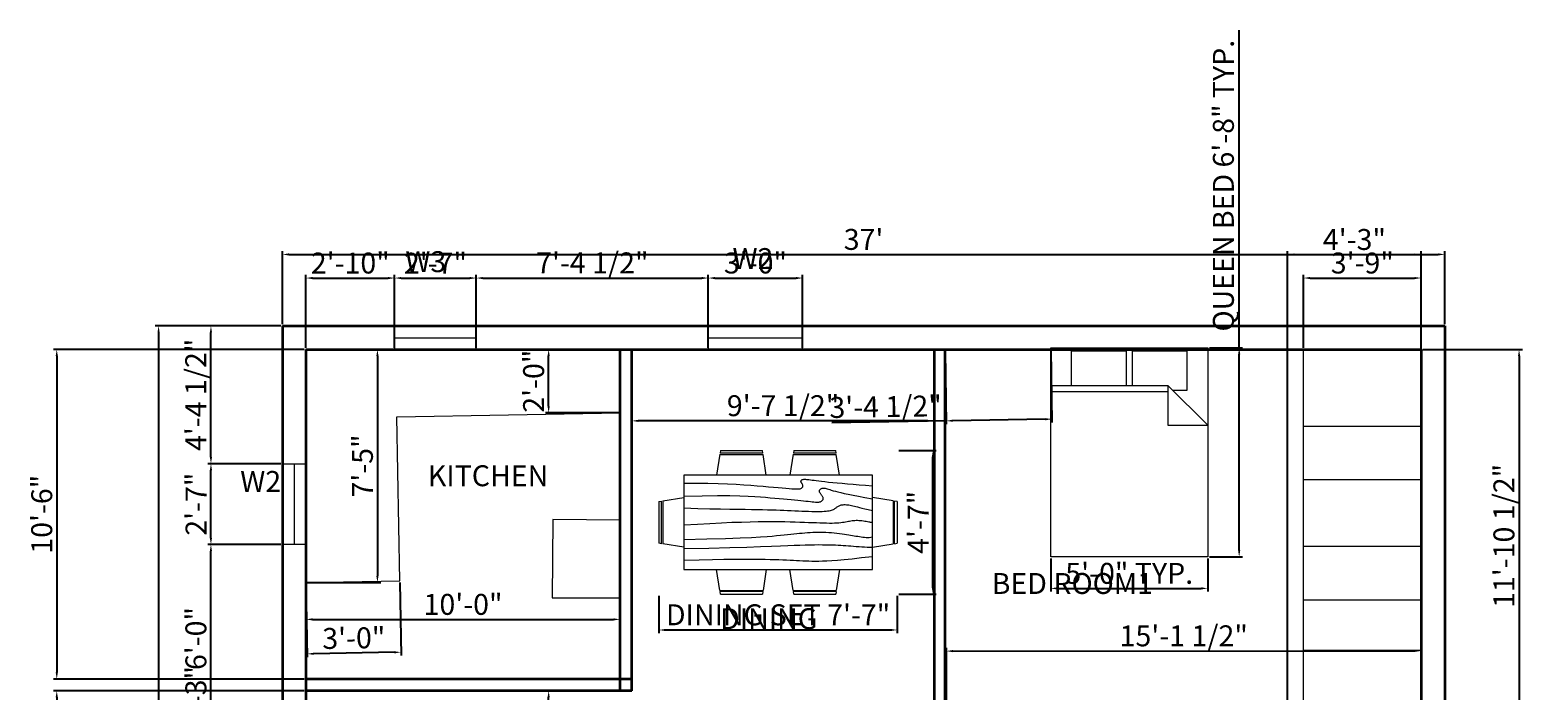
# Model space of a CAD drawing. Units: inches. Extents: x 56 to 631, y 587 to 1198.
# Tile 3 of 3: x 56 to 631, y 946 to 1198. Entities that reach past the tile are written whole.
import ezdxf

# ---------------------------------------------------------------- set-up
doc = ezdxf.new("R2010")
doc.units = ezdxf.units.IN
for name, color, linetype, lineweight in [('A-ANNO-DIMS', 2, 'Continuous', 18), ('A-ANNO-TEXT', 7, 'Continuous', 18), ('A-AREA-IDEN', 7, 'Continuous', 25), ('A-FLOR-CASE', 9, 'Continuous', 18), ('A-FURN', 8, 'Continuous', 18), ('A-GLAZ', 4, 'Continuous', 18), ('WALL', 7, 'Continuous', 35)]:
    doc.layers.add(name, color=color, linetype=linetype, lineweight=lineweight)
doc.styles.get("Standard").update_dxf_attribs({"font": 'arial.ttf', "height": 8})
doc.dimstyles.new('ISO-25', dxfattribs={"dimtxt": 2.5, "dimasz": 2.5, "dimexe": 1.25, "dimexo": 0.625, "dimtad": 1, "dimdec": 1, "dimlunit": 3, "dimtxsty": 'Standard', "dimcen": 2.5, "dimadec": 0, "dimazin": 0, "dimtfac": 1, "dimtdec": 1, "dimtmove": 0, "dimatfit": 3, "dimfxl": 1, "dimarcsym": 0})

# ---------------------------------------------------------------- blocks, each defined once
blk = doc.blocks.new('Dining Set - 36 x 72 in.')
for p, q in [((-22.2343, 26.00059), (-23.4847, 17.99762)), ((-22.2304, 26), (-5.7608, 26)), ((-22, 27.5), (-22.1562, 26.50042)), ((-5.8416, 26.5), (-22.1534, 26.5)), ((-22, 27.5), (-6, 27.5)), ((-5.8437, 26.49966), (-6, 27.5)), ((-4.5152, 17.99762), (-5.7655, 25.99926)), ((5.7657, 26.00059), (4.5153, 17.99762)), ((5.7696, 26), (22.2392, 26)), ((6, 27.5), (5.8438, 26.50042)), ((22.1584, 26.5), (5.8466, 26.5)), ((6, 27.5), (22, 27.5)), ((22.1563, 26.49966), (22, 27.5)), ((23.4848, 17.99762), (22.2345, 25.99926)), ((36, 18), (-36, 18)), ((-36, 18), (-36, -18)), ((36, -18), (36, 18)), ((-45.5, 8), (-44.5004, 8.15617)), ((-45.5, 8), (-45.5, -8)), ((-44.5, -8.15843), (-44.5, 8.15338)), ((-44.0006, 8.23428), (-35.9976, 9.48474)), ((-44, 8.23041), (-44, -8.23915)), ((44.0006, 8.23428), (35.9976, 9.48474)), ((44, 8.23041), (44, -8.23915)), ((44.5, -8.15843), (44.5, 8.15338)), ((45.5, 8), (44.5005, 8.15617)), ((45.5, 8), (45.5, -8)), ((-44.4997, -8.15631), (-45.5, -8)), ((-35.9976, -9.48476), (-43.9993, -8.2345)), ((35.9976, -9.48476), (43.9993, -8.2345)), ((44.4997, -8.15631), (45.5, -8)), ((-36, -18), (36, -18)), ((-22.2343, -26.0006), (-23.4847, -17.99762)), ((-4.5152, -17.99762), (-5.7655, -25.99928)), ((5.7657, -26.0006), (4.5153, -17.99762)), ((23.4848, -17.99762), (22.2345, -25.99928)), ((-22.2304, -26), (-5.7608, -26)), ((-22, -27.5), (-22.1562, -26.50044)), ((-5.8416, -26.5), (-22.1534, -26.5)), ((-22, -27.5), (-6, -27.5)), ((-5.8437, -26.49967), (-6, -27.5)), ((5.7696, -26), (22.2392, -26)), ((6, -27.5), (5.8438, -26.50044)), ((22.1584, -26.5), (5.8466, -26.5)), ((6, -27.5), (22, -27.5)), ((22.1563, -26.49967), (22, -27.5))]:
    blk.add_line(p, q)
for points in [[(-36, 15), (-31.1772, 14.97754), (-26.8079, 14.91406), (-22.8538, 14.81543), (-19.276, 14.6875), (-16.0362, 14.53613), (-13.0957, 14.36718), (-10.4159, 14.18652), (-7.9583, 14), (-5.6904, 13.81315), (-3.6035, 13.63021), (-1.6954, 13.45508), (0.0365, 13.29166), (1.5945, 13.14388), (2.9811, 13.01562), (4.1988, 12.9108), (5.25, 12.83333), (6.1393, 12.78613), (6.8802, 12.76823), (7.4883, 12.77767), (7.9792, 12.8125), (8.3685, 12.87077), (8.6719, 12.95052), (8.9049, 13.0498), (9.0833, 13.16666), (9.2205, 13.29899), (9.3216, 13.44401), (9.3895, 13.59879), (9.4271, 13.76041), (9.4373, 13.92594), (9.4232, 14.09245), (9.3875, 14.257), (9.3333, 14.41666), (9.2638, 14.56917), (9.1836, 14.71484), (9.0975, 14.85465), (9.0104, 14.98958), (8.9272, 15.1206), (8.8529, 15.2487), (8.7922, 15.37483), (8.75, 15.5), (8.7305, 15.62467), (8.7344, 15.74739), (8.7617, 15.86621), (8.8125, 15.97916), (8.8867, 16.08431), (8.9844, 16.17968), (9.1055, 16.26334), (9.25, 16.33333), (9.4189, 16.38802), (9.6172, 16.42708), (9.8506, 16.45052), (10.125, 16.45833), (10.4463, 16.45052), (10.8203, 16.42708), (11.2529, 16.38802), (11.75, 16.33333), (12.3184, 16.26318), (12.9694, 16.17838), (13.7151, 16.07991), (14.5677, 15.96875), (15.5395, 15.84586), (16.6426, 15.71224), (17.8893, 15.56884), (19.2917, 15.41666), (20.859, 15.25667), (22.5879, 15.08984), (24.4721, 14.91715), (26.5052, 14.73958), (28.6809, 14.5581), (30.9929, 14.3737), (33.4347, 14.18733), (36, 14)], [(-36, 10), (-28.9766, 10.14274), (-23.1725, 10.20442), (-18.4241, 10.19775), (-14.5677, 10.13541), (-11.4399, 10.03011), (-8.877, 9.89453), (-6.7154, 9.74137), (-4.7917, 9.58333), (-2.9698, 9.43082), (-1.2246, 9.28515), (0.4415, 9.14534), (2.026, 9.01041), (3.5266, 8.87939), (4.9408, 8.7513), (6.266, 8.62516), (7.5, 8.5), (8.6411, 8.37549), (9.6914, 8.2539), (10.6538, 8.13818), (11.5312, 8.03125), (12.3267, 7.93603), (13.043, 7.85547), (13.6831, 7.79248), (14.25, 7.75), (14.7471, 7.7303), (15.1797, 7.73307), (15.5537, 7.75732), (15.875, 7.80208), (16.1494, 7.86637), (16.3828, 7.94922), (16.5811, 8.04964), (16.75, 8.16666), (16.8944, 8.29915), (17.0143, 8.44531), (17.1089, 8.60319), (17.1771, 8.77083), (17.218, 8.94629), (17.2305, 9.1276), (17.2137, 9.31282), (17.1667, 9.5), (17.0895, 9.6875), (16.987, 9.875), (16.8649, 10.0625), (16.7292, 10.25), (16.5856, 10.4375), (16.4401, 10.625), (16.2985, 10.8125), (16.1667, 11), (16.05, 11.18733), (15.9518, 11.3737), (15.8752, 11.5581), (15.8229, 11.73958), (15.798, 11.91715), (15.8034, 12.08984), (15.842, 12.25667), (15.9167, 12.41666), (16.0295, 12.56836), (16.1784, 12.70833), (16.3605, 12.83268), (16.5729, 12.9375), (16.8127, 13.01888), (17.0768, 13.07291), (17.3625, 13.0957), (17.6667, 13.08333), (17.9894, 13.03312), (18.3418, 12.94726), (18.7382, 12.82918), (19.1927, 12.68229), (19.7195, 12.51001), (20.3327, 12.31575), (21.0465, 12.10294), (21.875, 11.875), (22.8357, 11.63354), (23.959, 11.37304), (25.2786, 11.08618), (26.8282, 10.76562), (28.6414, 10.40405), (30.752, 9.99414), (33.1936, 9.52856), (36, 9)], [(-36, 5.5), (-30.7157, 5.3348), (-26.069, 5.20963), (-21.9946, 5.11767), (-18.4271, 5.05208), (-15.3009, 5.00602), (-12.5508, 4.97265), (-10.1112, 4.94515), (-7.9167, 4.91666), (-5.909, 4.88167), (-4.0586, 4.83984), (-2.3429, 4.79215), (-0.7396, 4.73958), (0.7739, 4.6831), (2.22, 4.6237), (3.6213, 4.56233), (5, 4.5), (6.373, 4.43782), (7.7344, 4.3776), (9.0723, 4.32129), (10.375, 4.27083), (11.6309, 4.22819), (12.8281, 4.19531), (13.9551, 4.17415), (15, 4.16666), (15.954, 4.17448), (16.819, 4.19791), (17.6001, 4.23698), (18.3021, 4.29166), (18.9299, 4.36198), (19.4883, 4.44791), (19.9823, 4.54948), (20.4167, 4.66666), (20.7969, 4.79899), (21.1302, 4.94401), (21.4245, 5.09879), (21.6875, 5.26041), (21.9271, 5.42594), (22.1511, 5.59245), (22.3672, 5.757), (22.5834, 5.91666), (22.8065, 6.06868), (23.0404, 6.21093), (23.2879, 6.34147), (23.5521, 6.45833), (23.8358, 6.55957), (24.142, 6.64323), (24.4735, 6.70735), (24.8334, 6.75), (25.2235, 6.76969), (25.642, 6.76692), (26.0858, 6.74267), (26.5521, 6.69791), (27.0379, 6.63362), (27.5404, 6.55078), (28.0565, 6.45036), (28.5834, 6.33333), (29.1242, 6.19987), (29.7071, 6.04687), (30.3661, 5.87044), (31.1354, 5.66666), (32.0493, 5.43164), (33.142, 5.16146), (34.4475, 4.85221), (36, 4.5)], [(-36, -1), (-30.7915, -0.6591), (-26.0195, -0.38216), (-21.6519, -0.16284), (-17.6563, 0.00521), (-14.0005, 0.12833), (-10.6523, 0.21289), (-7.5796, 0.26522), (-4.75, 0.29166), (-2.134, 0.29793), (0.2878, 0.28711), (2.5317, 0.26163), (4.6146, 0.22396), (6.5529, 0.17651), (8.3633, 0.12174), (10.0623, 0.06209), (11.6667, 0), (13.1899, -0.06201), (14.6341, -0.1211), (15.9982, -0.17432), (17.2813, -0.21875), (18.4823, -0.25147), (19.6003, -0.26953), (20.6343, -0.27002), (21.5834, -0.25), (22.4481, -0.20768), (23.2357, -0.14584), (23.9549, -0.06836), (24.6146, 0.02083), (25.2235, 0.11784), (25.7904, 0.21875), (26.3241, 0.31966), (26.8334, 0.41666), (27.3265, 0.50618), (27.8099, 0.58593), (28.2894, 0.65397), (28.7709, 0.70833), (29.2601, 0.74707), (29.763, 0.76823), (30.2855, 0.76985), (30.8334, 0.75), (31.4088, 0.70784), (31.9994, 0.64713), (32.589, 0.57275), (33.1615, 0.48958), (33.7008, 0.4025), (34.1908, 0.3164), (34.6153, 0.23616), (34.9584, 0.16666), (35.2099, 0.11165), (35.3848, 0.07031), (35.504, 0.04069), (35.5886, 0.02083), (35.6594, 0.00879), (35.7377, 0.0026), (35.8442, 0.00032), (36, 0)], [(-36, -6.5), (-27.1843, -6.31267), (-20.084, -6.1263), (-14.469, -5.9419), (-10.1094, -5.76042), (-6.7752, -5.58285), (-4.2363, -5.41016), (-2.2629, -5.24333), (-0.625, -5.08334), (0.8708, -4.93099), (2.2715, -4.78646), (3.5872, -4.64974), (4.8281, -4.52084), (6.0046, -4.39974), (7.127, -4.28646), (8.2053, -4.18099), (9.25, -4.08334), (10.2705, -3.99382), (11.2734, -3.91407), (12.2647, -3.84603), (13.25, -3.79167), (14.2354, -3.75293), (15.2266, -3.73177), (16.2295, -3.73015), (17.25, -3.75), (18.2912, -3.79248), (19.3451, -3.85547), (20.4009, -3.93604), (21.4479, -4.03125), (22.4754, -4.13819), (23.4727, -4.25391), (24.4289, -4.37549), (25.3334, -4.5), (26.1785, -4.62492), (26.9694, -4.74935), (27.7145, -4.87281), (28.4219, -4.99479), (29.1, -5.11483), (29.7572, -5.23242), (30.4016, -5.34709), (31.0417, -5.45834), (31.6837, -5.56437), (32.3262, -5.65821), (32.9658, -5.73153), (33.599, -5.77604), (34.2224, -5.78345), (34.8327, -5.74545), (35.4264, -5.65373), (36, -5.5)], [(-36, -10), (-26.4022, -9.81299), (-18.4675, -9.62891), (-11.9839, -9.45069), (-6.7396, -9.28125), (-2.5226, -9.12354), (0.8789, -8.98047), (3.6769, -8.85498), (6.0833, -8.75), (8.2767, -8.66765), (10.3021, -8.60677), (12.1712, -8.56543), (13.8958, -8.54167), (15.4876, -8.53353), (16.9583, -8.53907), (18.3197, -8.55632), (19.5834, -8.58334), (20.7616, -8.61841), (21.8685, -8.66081), (22.9188, -8.71004), (23.9271, -8.76563), (24.9081, -8.82707), (25.8763, -8.89388), (26.8465, -8.96558), (27.8334, -9.04167), (28.8474, -9.12118), (29.8828, -9.20117), (30.93, -9.27824), (31.9792, -9.34896), (33.0205, -9.40991), (34.0443, -9.45768), (35.0407, -9.48885), (36, -9.5)], [(-36, -14.5), (-30.0881, -14.33513), (-25.0332, -14.21224), (-20.7312, -14.12647), (-17.0781, -14.07292), (-13.97, -14.04671), (-11.3027, -14.04297), (-8.9724, -14.05681), (-6.875, -14.08334), (-4.9224, -14.11833), (-3.0905, -14.16016), (-1.3709, -14.20785), (0.2448, -14.26042), (1.7647, -14.3169), (3.1973, -14.3763), (4.5507, -14.43767), (5.8333, -14.5), (7.0554, -14.5621), (8.235, -14.62175), (9.3922, -14.67652), (10.5469, -14.72396), (11.7192, -14.76164), (12.929, -14.78711), (14.1965, -14.79794), (15.5417, -14.79167), (16.9933, -14.76424), (18.6152, -14.70508), (20.4804, -14.60197), (22.6615, -14.44271), (25.2312, -14.21509), (28.2624, -13.9069), (31.8277, -13.50594), (36, -13)]]:
    blk.add_lwpolyline(points)
blk = doc.blocks.new('Bed - Queen')
for p, q in [((0, -80.00003), (0, 0)), ((0, 0), (59.99999, 0)), ((59.99999, 0), (59.99999, -80.00003)), ((7.99999, -1.2), (28.79998, -1.2)), ((7.99999, -14.4), (7.99999, -1.2)), ((28.79998, -1.2), (28.79998, -14.4)), ((31.19999, -1.2), (51.99999, -1.2)), ((31.19999, -14.4), (31.19999, -1.2)), ((51.99999, -1.2), (51.99999, -16.4)), ((0, -14.4), (44.8, -14.4)), ((44.8, -16.8), (0, -16.8)), ((59.99999, -29.6), (44.8, -14.4)), ((44.8, -14.4), (44.8, -29.6)), ((51.99999, -16.4), (46.79936, -16.4)), ((44.8, -29.6), (59.99999, -29.6)), ((59.99999, -80.00003), (0, -80.00003))]:
    blk.add_line(p, q)
blk = doc.blocks.new('*D11')
at = {"layer": 'A-ANNO-DIMS', "color": 0, "lineweight": -2, "transparency": 16777216}
for p, q in [((151.92, 1085.91), (151.92, 1113.87)), ((154.42, 1112.62), (593.42, 1112.62)), ((595.92, 1085.91), (595.92, 1113.87))]:
    blk.add_line(p, q, dxfattribs=at)
at = {"layer": 'A-ANNO-DIMS', "color": 0, "transparency": 16777216}
for points in [[(154.42, 1113.04), (154.42, 1112.2), (151.92, 1112.62)], [(593.42, 1113.04), (593.42, 1112.2), (595.92, 1112.62)]]:
    blk.add_solid(points, dxfattribs=at)
at = {"layer": 'Defpoints', "color": 0, "transparency": 16777216}
for p in [(595.92, 1112.62), (151.92, 1085.29), (595.92, 1085.29)]:
    blk.add_point(p, dxfattribs=at)
at = {"layer": 'A-ANNO-DIMS', "color": 0, "transparency": 16777216, "insert": (373.92, 1117.33), "char_height": 8, "attachment_point": 5}
blk.add_mtext("37'", dxfattribs=at)
blk = doc.blocks.new('*D12')
at = {"layer": 'A-ANNO-DIMS', "color": 0, "lineweight": -2, "transparency": 16777216}
for p, q in [((151.29, 1085.29), (103.37, 1085.29)), ((104.62, 1082.79), (104.62, 624.29)), ((151.29, 621.79), (103.37, 621.79))]:
    blk.add_line(p, q, dxfattribs=at)
at = {"layer": 'A-ANNO-DIMS', "color": 0, "transparency": 16777216}
for points in [[(104.2, 1082.79), (105.03, 1082.79), (104.62, 1085.29)], [(104.2, 624.29), (105.03, 624.29), (104.62, 621.79)]]:
    blk.add_solid(points, dxfattribs=at)
at = {"layer": 'Defpoints', "color": 0, "transparency": 16777216}
for p in [(151.92, 1085.29), (104.62, 621.79), (151.92, 621.79)]:
    blk.add_point(p, dxfattribs=at)
at = {"layer": 'A-ANNO-DIMS', "color": 0, "transparency": 16777216, "insert": (99.9, 853.54), "char_height": 8, "attachment_point": 5, "rotation": 90}
blk.add_mtext('38\'-7.5"', dxfattribs=at)
blk = doc.blocks.new('*D13')
at = {"layer": 'A-ANNO-DIMS', "color": 0, "lineweight": -2, "transparency": 16777216}
for p, q in [((517.4, 1076.94), (517.4, 1198.37)), ((506.03, 1076.94), (518.65, 1076.94)), ((517.4, 999.44), (517.4, 1074.44)), ((506.03, 996.94), (518.65, 996.94))]:
    blk.add_line(p, q, dxfattribs=at)
at = {"layer": 'A-ANNO-DIMS', "color": 0, "transparency": 16777216}
for points in [[(516.99, 1074.44), (517.82, 1074.44), (517.4, 1076.94)], [(516.99, 999.44), (517.82, 999.44), (517.4, 996.94)]]:
    blk.add_solid(points, dxfattribs=at)
at = {"layer": 'Defpoints', "color": 0, "transparency": 16777216}
for p in [(505.4, 1076.94), (517.4, 1076.94), (505.4, 996.94)]:
    blk.add_point(p, dxfattribs=at)
at = {"layer": 'A-ANNO-DIMS', "color": 0, "transparency": 16777216, "insert": (512.4, 1138.91), "char_height": 8, "attachment_point": 5, "rotation": 90}
blk.add_mtext('QUEEN BED 6\'-8" TYP.', dxfattribs=at)
blk = doc.blocks.new('*D14')
at = {"layer": 'A-ANNO-DIMS', "color": 0, "lineweight": -2, "transparency": 16777216}
for p, q in [((445.4, 996.32), (445.4, 983.69)), ((505.4, 996.32), (505.4, 983.69)), ((447.9, 984.94), (502.9, 984.94))]:
    blk.add_line(p, q, dxfattribs=at)
at = {"layer": 'A-ANNO-DIMS', "color": 0, "transparency": 16777216}
for points in [[(447.9, 985.36), (447.9, 984.53), (445.4, 984.94)], [(502.9, 985.36), (502.9, 984.53), (505.4, 984.94)]]:
    blk.add_solid(points, dxfattribs=at)
at = {"layer": 'Defpoints', "color": 0, "transparency": 16777216}
for p in [(445.4, 996.94), (505.4, 996.94), (505.4, 984.94)]:
    blk.add_point(p, dxfattribs=at)
at = {"layer": 'A-ANNO-DIMS', "color": 0, "transparency": 16777216, "insert": (475.4, 989.65), "char_height": 8, "attachment_point": 5}
blk.add_mtext('5\'-0" TYP.', dxfattribs=at)
blk = doc.blocks.new('*D15')
at = {"layer": 'A-ANNO-DIMS', "color": 0, "lineweight": -2, "transparency": 16777216}
for p, q in [((295.77, 982.06), (295.77, 967.79)), ((386.77, 982.06), (386.77, 967.79)), ((298.27, 969.04), (384.27, 969.04))]:
    blk.add_line(p, q, dxfattribs=at)
at = {"layer": 'A-ANNO-DIMS', "color": 0, "transparency": 16777216}
for points in [[(298.27, 969.45), (298.27, 968.62), (295.77, 969.04)], [(384.27, 969.45), (384.27, 968.62), (386.77, 969.04)]]:
    blk.add_solid(points, dxfattribs=at)
at = {"layer": 'Defpoints', "color": 0, "transparency": 16777216}
for p in [(295.77, 982.69), (386.77, 982.69), (386.77, 969.04)]:
    blk.add_point(p, dxfattribs=at)
at = {"layer": 'A-ANNO-DIMS', "color": 0, "transparency": 16777216, "insert": (341.27, 973.8), "char_height": 8, "attachment_point": 5}
blk.add_mtext('DINING SET 7\'-7"', dxfattribs=at)
blk = doc.blocks.new('*D16')
at = {"layer": 'A-ANNO-DIMS', "color": 0, "lineweight": -2, "transparency": 16777216}
for p, q in [((387.39, 1037.69), (401.67, 1037.69)), ((400.42, 985.19), (400.42, 1035.19)), ((387.39, 982.69), (401.67, 982.69))]:
    blk.add_line(p, q, dxfattribs=at)
at = {"layer": 'A-ANNO-DIMS', "color": 0, "transparency": 16777216}
for points in [[(400, 1035.19), (400.84, 1035.19), (400.42, 1037.69)], [(400, 985.19), (400.84, 985.19), (400.42, 982.69)]]:
    blk.add_solid(points, dxfattribs=at)
at = {"layer": 'Defpoints', "color": 0, "transparency": 16777216}
for p in [(386.77, 1037.69), (400.42, 1037.69), (386.77, 982.69)]:
    blk.add_point(p, dxfattribs=at)
at = {"layer": 'A-ANNO-DIMS', "color": 0, "transparency": 16777216, "insert": (395.79, 1010.19), "char_height": 8, "attachment_point": 5, "rotation": 90}
blk.add_mtext('4\'-7"', dxfattribs=at)
blk = doc.blocks.new('*D22')
at = {"layer": 'A-ANNO-DIMS', "color": 0, "lineweight": -2, "transparency": 16777216}
for p, q in [((160.92, 946.41), (160.92, 974.34)), ((280.92, 946.41), (280.92, 974.34)), ((163.42, 973.09), (278.42, 973.09))]:
    blk.add_line(p, q, dxfattribs=at)
at = {"layer": 'A-ANNO-DIMS', "color": 0, "transparency": 16777216}
for points in [[(163.42, 973.5), (163.42, 972.67), (160.92, 973.09)], [(278.42, 973.5), (278.42, 972.67), (280.92, 973.09)]]:
    blk.add_solid(points, dxfattribs=at)
at = {"layer": 'Defpoints', "color": 0, "transparency": 16777216}
for p in [(280.92, 973.09), (160.92, 945.79), (280.92, 945.79)]:
    blk.add_point(p, dxfattribs=at)
at = {"layer": 'A-ANNO-DIMS', "color": 0, "transparency": 16777216, "insert": (220.92, 977.79), "char_height": 8, "attachment_point": 5}
blk.add_mtext('10\'-0"', dxfattribs=at)
blk = doc.blocks.new('*D23')
at = {"layer": 'A-ANNO-DIMS', "color": 0, "lineweight": -2, "transparency": 16777216}
for p, q in [((285.42, 1075.66), (285.42, 1047.74)), ((400.92, 1075.66), (400.92, 1047.74)), ((398.42, 1048.99), (287.92, 1048.99))]:
    blk.add_line(p, q, dxfattribs=at)
at = {"layer": 'A-ANNO-DIMS', "color": 0, "transparency": 16777216}
for points in [[(287.92, 1049.4), (287.92, 1048.57), (285.42, 1048.99)], [(398.42, 1049.4), (398.42, 1048.57), (400.92, 1048.99)]]:
    blk.add_solid(points, dxfattribs=at)
at = {"layer": 'Defpoints', "color": 0, "transparency": 16777216}
for p in [(285.42, 1076.29), (400.92, 1076.29), (285.42, 1048.99)]:
    blk.add_point(p, dxfattribs=at)
at = {"layer": 'A-ANNO-DIMS', "color": 0, "transparency": 16777216, "insert": (343.17, 1053.75), "char_height": 8, "attachment_point": 5}
blk.add_mtext('9\'-7 1/2"', dxfattribs=at)
blk = doc.blocks.new('*D24')
at = {"layer": 'A-ANNO-DIMS', "color": 0, "lineweight": -2, "transparency": 16777216}
for p, q in [((405.55, 934.28), (405.54, 962.2)), ((586.91, 934.37), (586.9, 962.3)), ((408.04, 960.95), (584.4, 961.04))]:
    blk.add_line(p, q, dxfattribs=at)
at = {"layer": 'A-ANNO-DIMS', "color": 0, "transparency": 16777216}
for points in [[(408.04, 961.37), (408.04, 960.54), (405.54, 960.95)], [(584.4, 961.46), (584.4, 960.63), (586.9, 961.05)]]:
    blk.add_solid(points, dxfattribs=at)
at = {"layer": 'Defpoints', "color": 0, "transparency": 16777216}
for p in [(586.9, 961.05), (405.55, 933.65), (586.92, 933.75)]:
    blk.add_point(p, dxfattribs=at)
at = {"layer": 'A-ANNO-DIMS', "color": 0, "transparency": 16777216, "insert": (496.22, 965.76), "char_height": 8, "attachment_point": 5, "rotation": 0.02972}
blk.add_mtext('15\'-1 1/2"', dxfattribs=at)
blk = doc.blocks.new('*D26')
at = {"layer": 'A-ANNO-DIMS', "color": 0, "lineweight": -2, "transparency": 16777216}
for p, q in [((535.92, 796.41), (535.92, 1113.84)), ((538.42, 1112.59), (584.42, 1112.59)), ((586.92, 796.41), (586.92, 1113.84))]:
    blk.add_line(p, q, dxfattribs=at)
at = {"layer": 'A-ANNO-DIMS', "color": 0, "transparency": 16777216}
for points in [[(538.42, 1113), (538.42, 1112.17), (535.92, 1112.59)], [(584.42, 1113), (584.42, 1112.17), (586.92, 1112.59)]]:
    blk.add_solid(points, dxfattribs=at)
at = {"layer": 'Defpoints', "color": 0, "transparency": 16777216}
for p in [(586.92, 1112.59), (535.92, 795.79), (586.92, 795.79)]:
    blk.add_point(p, dxfattribs=at)
at = {"layer": 'A-ANNO-DIMS', "color": 0, "transparency": 16777216, "insert": (561.42, 1117.3), "char_height": 8, "attachment_point": 5}
blk.add_mtext('4\'-3"', dxfattribs=at)
blk = doc.blocks.new('*D27')
at = {"layer": 'A-ANNO-DIMS', "color": 0, "lineweight": -2, "transparency": 16777216}
for p, q in [((160.29, 1076.29), (64.47, 1076.29)), ((65.72, 1073.79), (65.72, 952.79)), ((160.29, 950.29), (64.47, 950.29))]:
    blk.add_line(p, q, dxfattribs=at)
at = {"layer": 'A-ANNO-DIMS', "color": 0, "transparency": 16777216}
for points in [[(65.31, 1073.79), (66.14, 1073.79), (65.72, 1076.29)], [(65.31, 952.79), (66.14, 952.79), (65.72, 950.29)]]:
    blk.add_solid(points, dxfattribs=at)
at = {"layer": 'Defpoints', "color": 0, "transparency": 16777216}
for p in [(160.92, 1076.29), (65.72, 950.29), (160.92, 950.29)]:
    blk.add_point(p, dxfattribs=at)
at = {"layer": 'A-ANNO-DIMS', "color": 0, "transparency": 16777216, "insert": (61.01, 1013.29), "char_height": 8, "attachment_point": 5, "rotation": 90}
blk.add_mtext('10\'-6"', dxfattribs=at)
blk = doc.blocks.new('*D28')
at = {"layer": 'A-ANNO-DIMS', "color": 0, "lineweight": -2, "transparency": 16777216}
for p, q in [((160.29, 945.79), (64.47, 945.79)), ((65.72, 943.29), (65.72, 900.29)), ((160.29, 897.79), (64.47, 897.79))]:
    blk.add_line(p, q, dxfattribs=at)
at = {"layer": 'A-ANNO-DIMS', "color": 0, "transparency": 16777216}
for points in [[(65.31, 943.29), (66.14, 943.29), (65.72, 945.79)], [(65.31, 900.29), (66.14, 900.29), (65.72, 897.79)]]:
    blk.add_solid(points, dxfattribs=at)
at = {"layer": 'Defpoints', "color": 0, "transparency": 16777216}
for p in [(160.92, 945.79), (65.72, 897.79), (160.92, 897.79)]:
    blk.add_point(p, dxfattribs=at)
at = {"layer": 'A-ANNO-DIMS', "color": 0, "transparency": 16777216, "insert": (61.01, 921.79), "char_height": 8, "attachment_point": 5, "rotation": 90}
blk.add_mtext('4\'-0"', dxfattribs=at)
blk = doc.blocks.new('*D30')
at = {"layer": 'A-ANNO-DIMS', "color": 0, "lineweight": -2, "transparency": 16777216}
for p, q in [((587.54, 1076.29), (625.57, 1076.29)), ((624.32, 1073.79), (624.32, 936.25)), ((587.54, 933.75), (625.57, 933.75))]:
    blk.add_line(p, q, dxfattribs=at)
at = {"layer": 'A-ANNO-DIMS', "color": 0, "transparency": 16777216}
for points in [[(623.9, 1073.79), (624.74, 1073.79), (624.32, 1076.29)], [(623.9, 936.25), (624.74, 936.25), (624.32, 933.75)]]:
    blk.add_solid(points, dxfattribs=at)
at = {"layer": 'Defpoints', "color": 0, "transparency": 16777216}
for p in [(586.92, 1076.29), (586.92, 933.75), (624.32, 933.75)]:
    blk.add_point(p, dxfattribs=at)
at = {"layer": 'A-ANNO-DIMS', "color": 0, "transparency": 16777216, "insert": (619.56, 1005.02), "char_height": 8, "attachment_point": 5, "rotation": 90}
blk.add_mtext('11\'-10 1/2"', dxfattribs=at)
blk = doc.blocks.new('*D33')
at = {"layer": 'A-ANNO-DIMS', "color": 0, "lineweight": -2, "transparency": 16777216}
for p, q in [((160.92, 1076.91), (160.92, 1104.84)), ((163.42, 1103.59), (192.28, 1103.59)), ((194.78, 1076.91), (194.78, 1104.84))]:
    blk.add_line(p, q, dxfattribs=at)
at = {"layer": 'A-ANNO-DIMS', "color": 0, "transparency": 16777216}
for points in [[(163.42, 1104), (163.42, 1103.17), (160.92, 1103.59)], [(192.28, 1104), (192.28, 1103.17), (194.78, 1103.59)]]:
    blk.add_solid(points, dxfattribs=at)
at = {"layer": 'Defpoints', "color": 0, "transparency": 16777216}
for p in [(194.78, 1103.59), (160.92, 1076.29), (194.78, 1076.29)]:
    blk.add_point(p, dxfattribs=at)
at = {"layer": 'A-ANNO-DIMS', "color": 0, "transparency": 16777216, "insert": (177.85, 1108.29), "char_height": 8, "attachment_point": 5}
blk.add_mtext('2\'-10"', dxfattribs=at)
blk = doc.blocks.new('*D34')
at = {"layer": 'A-ANNO-DIMS', "color": 0, "lineweight": -2, "transparency": 16777216}
for p, q in [((194.78, 1076.91), (194.78, 1104.84)), ((197.28, 1103.59), (223.48, 1103.59)), ((225.98, 1076.91), (225.98, 1104.84))]:
    blk.add_line(p, q, dxfattribs=at)
at = {"layer": 'A-ANNO-DIMS', "color": 0, "transparency": 16777216}
for points in [[(197.28, 1104), (197.28, 1103.17), (194.78, 1103.59)], [(223.48, 1104), (223.48, 1103.17), (225.98, 1103.59)]]:
    blk.add_solid(points, dxfattribs=at)
at = {"layer": 'Defpoints', "color": 0, "transparency": 16777216}
for p in [(225.98, 1103.59), (194.78, 1076.29), (225.98, 1076.29)]:
    blk.add_point(p, dxfattribs=at)
at = {"layer": 'A-ANNO-DIMS', "color": 0, "transparency": 16777216, "insert": (210.38, 1108.23), "char_height": 8, "attachment_point": 5}
blk.add_mtext('2\'-7"', dxfattribs=at)
blk = doc.blocks.new('*D35')
at = {"layer": 'A-ANNO-DIMS', "color": 0, "lineweight": -2, "transparency": 16777216}
for p, q in [((225.98, 1076.91), (225.98, 1104.84)), ((228.48, 1103.59), (312.12, 1103.59)), ((314.62, 1076.91), (314.62, 1104.84))]:
    blk.add_line(p, q, dxfattribs=at)
at = {"layer": 'A-ANNO-DIMS', "color": 0, "transparency": 16777216}
for points in [[(228.48, 1104), (228.48, 1103.17), (225.98, 1103.59)], [(312.12, 1104), (312.12, 1103.17), (314.62, 1103.59)]]:
    blk.add_solid(points, dxfattribs=at)
at = {"layer": 'Defpoints', "color": 0, "transparency": 16777216}
for p in [(314.62, 1103.59), (225.98, 1076.29), (314.62, 1076.29)]:
    blk.add_point(p, dxfattribs=at)
at = {"layer": 'A-ANNO-DIMS', "color": 0, "transparency": 16777216, "insert": (270.3, 1108.35), "char_height": 8, "attachment_point": 5}
blk.add_mtext('7\'-4 1/2"', dxfattribs=at)
blk = doc.blocks.new('*D36')
at = {"layer": 'A-ANNO-DIMS', "color": 0, "lineweight": -2, "transparency": 16777216}
for p, q in [((314.62, 1076.91), (314.62, 1104.84)), ((317.12, 1103.59), (348.12, 1103.59)), ((350.62, 1076.91), (350.62, 1104.84))]:
    blk.add_line(p, q, dxfattribs=at)
at = {"layer": 'A-ANNO-DIMS', "color": 0, "transparency": 16777216}
for points in [[(317.12, 1104), (317.12, 1103.17), (314.62, 1103.59)], [(348.12, 1104), (348.12, 1103.17), (350.62, 1103.59)]]:
    blk.add_solid(points, dxfattribs=at)
at = {"layer": 'Defpoints', "color": 0, "transparency": 16777216}
for p in [(350.62, 1103.59), (314.62, 1076.29), (350.62, 1076.29)]:
    blk.add_point(p, dxfattribs=at)
at = {"layer": 'A-ANNO-DIMS', "color": 0, "transparency": 16777216, "insert": (332.62, 1108.3), "char_height": 8, "attachment_point": 5}
blk.add_mtext('3\'-0"', dxfattribs=at)
blk = doc.blocks.new('*D43')
at = {"layer": 'A-ANNO-DIMS', "color": 0, "lineweight": -2, "transparency": 16777216}
for p, q in [((151.29, 1085.29), (123.37, 1085.29)), ((124.62, 1035.11), (124.62, 1082.79)), ((151.29, 1032.61), (123.37, 1032.61))]:
    blk.add_line(p, q, dxfattribs=at)
at = {"layer": 'A-ANNO-DIMS', "color": 0, "transparency": 16777216}
for points in [[(124.2, 1082.79), (125.03, 1082.79), (124.62, 1085.29)], [(124.2, 1035.11), (125.03, 1035.11), (124.62, 1032.61)]]:
    blk.add_solid(points, dxfattribs=at)
at = {"layer": 'Defpoints', "color": 0, "transparency": 16777216}
for p in [(124.62, 1085.29), (151.92, 1085.29), (151.92, 1032.61)]:
    blk.add_point(p, dxfattribs=at)
at = {"layer": 'A-ANNO-DIMS', "color": 0, "transparency": 16777216, "insert": (119.85, 1058.95), "char_height": 8, "attachment_point": 5, "rotation": 90}
blk.add_mtext('4\'-4 1/2"', dxfattribs=at)
blk = doc.blocks.new('*D44')
at = {"layer": 'A-ANNO-DIMS', "color": 0, "lineweight": -2, "transparency": 16777216}
for p, q in [((151.29, 1032.61), (123.37, 1032.61)), ((124.62, 1004.2), (124.62, 1030.11)), ((151.29, 1001.7), (123.37, 1001.7))]:
    blk.add_line(p, q, dxfattribs=at)
at = {"layer": 'A-ANNO-DIMS', "color": 0, "transparency": 16777216}
for points in [[(124.2, 1030.11), (125.03, 1030.11), (124.62, 1032.61)], [(124.2, 1004.2), (125.03, 1004.2), (124.62, 1001.7)]]:
    blk.add_solid(points, dxfattribs=at)
at = {"layer": 'Defpoints', "color": 0, "transparency": 16777216}
for p in [(124.62, 1032.61), (151.92, 1032.61), (151.92, 1001.7)]:
    blk.add_point(p, dxfattribs=at)
at = {"layer": 'A-ANNO-DIMS', "color": 0, "transparency": 16777216, "insert": (119.97, 1017.15), "char_height": 8, "attachment_point": 5, "rotation": 90}
blk.add_mtext('2\'-7"', dxfattribs=at)
blk = doc.blocks.new('*D45')
at = {"layer": 'A-ANNO-DIMS', "color": 0, "lineweight": -2, "transparency": 16777216}
for p, q in [((151.29, 1001.7), (123.37, 1001.7)), ((124.62, 932.35), (124.62, 999.2)), ((151.29, 929.85), (123.37, 929.85))]:
    blk.add_line(p, q, dxfattribs=at)
at = {"layer": 'A-ANNO-DIMS', "color": 0, "transparency": 16777216}
for points in [[(124.2, 999.2), (125.03, 999.2), (124.62, 1001.7)], [(124.2, 932.35), (125.03, 932.35), (124.62, 929.85)]]:
    blk.add_solid(points, dxfattribs=at)
at = {"layer": 'Defpoints', "color": 0, "transparency": 16777216}
for p in [(124.62, 1001.7), (151.92, 1001.7), (151.92, 929.85)]:
    blk.add_point(p, dxfattribs=at)
at = {"layer": 'A-ANNO-DIMS', "color": 0, "transparency": 16777216, "insert": (119.91, 965.77), "char_height": 8, "attachment_point": 5, "rotation": 90}
blk.add_mtext('6\'-0"', dxfattribs=at)
blk = doc.blocks.new('*D46')
at = {"layer": 'A-ANNO-DIMS', "color": 0, "lineweight": -2, "transparency": 16777216}
for p, q in [((124.62, 929.85), (124.62, 954.11)), ((151.29, 929.85), (123.37, 929.85)), ((124.62, 917.53), (124.62, 927.35)), ((151.29, 915.03), (123.37, 915.03))]:
    blk.add_line(p, q, dxfattribs=at)
at = {"layer": 'A-ANNO-DIMS', "color": 0, "transparency": 16777216}
for points in [[(124.2, 927.35), (125.03, 927.35), (124.62, 929.85)], [(124.2, 917.53), (125.03, 917.53), (124.62, 915.03)]]:
    blk.add_solid(points, dxfattribs=at)
at = {"layer": 'Defpoints', "color": 0, "transparency": 16777216}
for p in [(124.62, 929.85), (151.92, 929.85), (151.92, 915.03)]:
    blk.add_point(p, dxfattribs=at)
at = {"layer": 'A-ANNO-DIMS', "color": 0, "transparency": 16777216, "insert": (119.9, 943.23), "char_height": 8, "attachment_point": 5, "rotation": 90}
blk.add_mtext('1\'-3"', dxfattribs=at)
blk = doc.blocks.new('*D60')
at = {"layer": 'A-ANNO-DIMS', "color": 0, "lineweight": -2, "transparency": 16777216}
for p, q in [((280.29, 945.79), (252.37, 945.79)), ((253.62, 906.28), (253.62, 943.29)), ((280.29, 903.78), (252.37, 903.78))]:
    blk.add_line(p, q, dxfattribs=at)
at = {"layer": 'A-ANNO-DIMS', "color": 0, "transparency": 16777216}
for points in [[(253.2, 943.29), (254.03, 943.29), (253.62, 945.79)], [(253.2, 906.28), (254.03, 906.28), (253.62, 903.78)]]:
    blk.add_solid(points, dxfattribs=at)
at = {"layer": 'Defpoints', "color": 0, "transparency": 16777216}
for p in [(253.62, 945.79), (280.92, 945.79), (280.92, 903.78)]:
    blk.add_point(p, dxfattribs=at)
at = {"layer": 'A-ANNO-DIMS', "color": 0, "transparency": 16777216, "insert": (248.9, 924.78), "char_height": 8, "attachment_point": 5, "rotation": 90}
blk.add_mtext('3\'-6"', dxfattribs=at)
blk = doc.blocks.new('*D72')
at = {"layer": 'A-ANNO-DIMS', "color": 0, "lineweight": -2, "transparency": 16777216}
for p, q in [((541.96, 1076.91), (541.96, 1104.84)), ((544.46, 1103.59), (584.42, 1103.59)), ((586.92, 1076.91), (586.92, 1104.84))]:
    blk.add_line(p, q, dxfattribs=at)
at = {"layer": 'A-ANNO-DIMS', "color": 0, "transparency": 16777216}
for points in [[(544.46, 1104), (544.46, 1103.17), (541.96, 1103.59)], [(584.42, 1104), (584.42, 1103.17), (586.92, 1103.59)]]:
    blk.add_solid(points, dxfattribs=at)
at = {"layer": 'Defpoints', "color": 0, "transparency": 16777216}
for p in [(586.92, 1103.59), (541.96, 1076.29), (586.92, 1076.29)]:
    blk.add_point(p, dxfattribs=at)
at = {"layer": 'A-ANNO-DIMS', "color": 0, "transparency": 16777216, "insert": (564.44, 1108.3), "char_height": 8, "attachment_point": 5}
blk.add_mtext('3\'-9"', dxfattribs=at)
blk = doc.blocks.new('*D73')
at = {"layer": 'A-ANNO-DIMS', "color": 0, "lineweight": -2, "transparency": 16777216}
for p, q in [((280.29, 1076.29), (252.37, 1076.29)), ((253.62, 1054.56), (253.62, 1073.79)), ((280.29, 1052.06), (252.37, 1052.06))]:
    blk.add_line(p, q, dxfattribs=at)
at = {"layer": 'A-ANNO-DIMS', "color": 0, "transparency": 16777216}
for points in [[(253.2, 1073.79), (254.03, 1073.79), (253.62, 1076.29)], [(253.2, 1054.56), (254.03, 1054.56), (253.62, 1052.06)]]:
    blk.add_solid(points, dxfattribs=at)
at = {"layer": 'Defpoints', "color": 0, "transparency": 16777216}
for p in [(253.62, 1076.29), (280.92, 1076.29), (280.92, 1052.06)]:
    blk.add_point(p, dxfattribs=at)
at = {"layer": 'A-ANNO-DIMS', "color": 0, "transparency": 16777216, "insert": (248.91, 1064.17), "char_height": 8, "attachment_point": 5, "rotation": 90}
blk.add_mtext('2\'-0"', dxfattribs=at)
blk = doc.blocks.new('*D74')
at = {"layer": 'A-ANNO-DIMS', "color": 0, "lineweight": -2, "transparency": 16777216}
for p, q in [((160.93, 986.57), (161.42, 958.65)), ((196.73, 987.2), (197.23, 959.28)), ((194.7, 960.49), (163.9, 959.94))]:
    blk.add_line(p, q, dxfattribs=at)
at = {"layer": 'A-ANNO-DIMS', "color": 0, "transparency": 16777216}
for points in [[(163.89, 960.36), (163.91, 959.53), (161.4, 959.9)], [(194.7, 960.91), (194.71, 960.07), (197.2, 960.53)]]:
    blk.add_solid(points, dxfattribs=at)
at = {"layer": 'Defpoints', "color": 0, "transparency": 16777216}
for p in [(160.92, 987.2), (196.72, 987.83), (161.4, 959.9)]:
    blk.add_point(p, dxfattribs=at)
at = {"layer": 'A-ANNO-DIMS', "color": 0, "transparency": 16777216, "insert": (179.22, 964.93), "char_height": 8, "attachment_point": 5, "rotation": 1.01408}
blk.add_mtext('3\'-0"', dxfattribs=at)
blk = doc.blocks.new('*D75')
at = {"layer": 'A-ANNO-DIMS', "color": 0, "lineweight": -2, "transparency": 16777216}
for p, q in [((161.54, 1076.29), (189.47, 1076.29)), ((188.22, 1073.79), (188.22, 989.7)), ((161.54, 987.2), (189.47, 987.2))]:
    blk.add_line(p, q, dxfattribs=at)
at = {"layer": 'A-ANNO-DIMS', "color": 0, "transparency": 16777216}
for points in [[(187.8, 1073.79), (188.63, 1073.79), (188.22, 1076.29)], [(187.8, 989.7), (188.63, 989.7), (188.22, 987.2)]]:
    blk.add_solid(points, dxfattribs=at)
at = {"layer": 'Defpoints', "color": 0, "transparency": 16777216}
for p in [(160.92, 1076.29), (160.92, 987.2), (188.22, 987.2)]:
    blk.add_point(p, dxfattribs=at)
at = {"layer": 'A-ANNO-DIMS', "color": 0, "transparency": 16777216, "insert": (183.52, 1031.74), "char_height": 8, "attachment_point": 5, "rotation": 90}
blk.add_mtext('7\'-5"', dxfattribs=at)
blk = doc.blocks.new('*D77')
at = {"layer": 'A-ANNO-DIMS', "color": 0, "lineweight": -2, "transparency": 16777216}
for p, q in [((405.07, 1075.66), (405.53, 1047.74)), ((445.41, 1076.32), (445.87, 1048.4)), ((405.51, 1048.99), (361.86, 1048.28)), ((443.35, 1049.61), (408.01, 1049.03))]:
    blk.add_line(p, q, dxfattribs=at)
at = {"layer": 'A-ANNO-DIMS', "color": 0, "transparency": 16777216}
for points in [[(408, 1049.45), (408.01, 1048.61), (405.51, 1048.99)], [(443.34, 1050.02), (443.36, 1049.19), (445.85, 1049.65)]]:
    blk.add_solid(points, dxfattribs=at)
at = {"layer": 'Defpoints', "color": 0, "transparency": 16777216}
for p in [(405.06, 1076.29), (445.4, 1076.94), (405.51, 1048.99)]:
    blk.add_point(p, dxfattribs=at)
at = {"layer": 'A-ANNO-DIMS', "color": 0, "transparency": 16777216, "insert": (382.36, 1053.38), "char_height": 8, "attachment_point": 5, "rotation": 0.93566}
blk.add_mtext('3\'-4 1/2"', dxfattribs=at)

msp = doc.modelspace()

# ---------------------------------------------------------------- linework, layer by layer
at = {"layer": 'A-FLOR-CASE'}
for p, q in [((541.96, 933.75), (541.96, 1076.29)), ((195.61, 1050.55), (280.92, 1052.06)), ((196.72, 987.83), (195.61, 1050.55)), ((541.96, 1047.01), (586.92, 1047.01)), ((541.96, 1026.53), (586.92, 1026.53)), ((255.16, 1011.22), (254.95, 981.36)), ((280.92, 1011.04), (255.16, 1011.22)), ((541.96, 1001.09), (586.92, 1001.09)), ((160.92, 987.2), (196.72, 987.83)), ((254.95, 981.36), (280.92, 981.36)), ((541.96, 980.61), (586.92, 980.61)), ((541.96, 961.37), (586.92, 961.37))]:
    msp.add_line(p, q, dxfattribs=at)
at = {"layer": 'A-GLAZ'}
for p, q in [((194.78, 1085.29), (194.78, 1076.29)), ((225.98, 1076.29), (225.98, 1085.29)), ((314.62, 1085.29), (314.62, 1076.29)), ((350.62, 1076.29), (350.62, 1085.29)), ((194.78, 1080.79), (225.98, 1080.79)), ((314.62, 1080.79), (350.62, 1080.79)), ((194.78, 1076.29), (225.98, 1076.29)), ((314.62, 1076.29), (350.62, 1076.29)), ((151.92, 1032.61), (160.92, 1032.61)), ((156.42, 1032.61), (156.42, 1001.7)), ((160.92, 1032.61), (160.92, 1001.7)), ((160.92, 1001.7), (151.92, 1001.7))]:
    msp.add_line(p, q, dxfattribs=at)
at = {"layer": 'WALL'}
for p, q in [((151.92, 1085.29), (151.92, 753.78)), ((151.92, 1085.29), (595.92, 1085.29)), ((595.92, 1085.29), (595.92, 621.79)), ((160.92, 1076.29), (586.92, 1076.29)), ((160.92, 1076.29), (160.92, 753.78)), ((280.92, 945.79), (280.92, 1076.29)), ((285.42, 945.79), (285.42, 1076.29)), ((400.92, 1076.29), (400.92, 933.75)), ((405.06, 933.78), (405.06, 1076.29)), ((586.92, 1076.29), (586.92, 711.79)), ((285.42, 950.29), (160.92, 950.29)), ((285.42, 945.79), (160.92, 945.79))]:
    msp.add_line(p, q, dxfattribs=at)

# ---------------------------------------------------------------- block references
at = {"layer": 'A-FURN'}
for name, p in [('Bed - Queen', (445.4, 1076.94)), ('Dining Set - 36 x 72 in.', (341.27, 1010.19))]:
    msp.add_blockref(name, p, dxfattribs=at)

# ---------------------------------------------------------------- texts
at = {"layer": 'A-ANNO-TEXT'}
for s, p in [('W3', (198.87, 1105.85)), ('W2', (323.85, 1107.02)), ('W2', (135.8, 1021.82))]:
    msp.add_text(s, height=8, dxfattribs=at).set_placement(p)
at = {"layer": 'A-AREA-IDEN'}
for s, p in [('KITCHEN', (207.47, 1024)), ('BED ROOM1', (422.85, 982.81)), ('DINING', (319.09, 969.36))]:
    msp.add_text(s, height=8, dxfattribs=at).set_placement(p)

# ---------------------------------------------------------------- dimensions: what is measured, and where the dimension line sits
at = {"layer": 'A-ANNO-DIMS'}
dim = msp.add_linear_dim(base=(517.4, 1076.94), p1=(505.4, 996.94), p2=(505.4, 1076.94), angle=90, text='QUEEN BED <> TYP.', dimstyle='ISO-25', override={"dimdec": 1, "dimlfac": 1, "dimrnd": 0, "dimzin": 1, "dimdsep": 46, "dimlunit": 4, "dimfrac": 2}, dxfattribs=at)
dim.commit()
dim.dimension.update_dxf_attribs({"geometry": '*D13', "text_midpoint": (512.4, 1138.91)})
for base, p1, p2, override, picture, middle in [((595.92, 1112.62), (151.92, 1085.29), (595.92, 1085.29), {"dimclrd": 0, "dimclre": 0, "dimclrt": 0}, '*D11', (373.92, 1117.33)), ((314.62, 1103.59), (225.98, 1076.29), (314.62, 1076.29), {"dimdec": 1, "dimlfac": 1, "dimrnd": 0, "dimzin": 1, "dimdsep": 46, "dimlunit": 4, "dimfrac": 2}, '*D35', (270.3, 1108.35)), ((586.92, 1112.59), (535.92, 795.79), (586.92, 795.79), {"dimdec": 1, "dimlfac": 1, "dimrnd": 0, "dimzin": 1, "dimdsep": 46, "dimlunit": 4, "dimfrac": 2}, '*D26', (561.42, 1117.3)), ((194.78, 1103.59), (160.92, 1076.29), (194.78, 1076.29), {"dimdec": 1, "dimlfac": 1, "dimrnd": 0, "dimzin": 1, "dimdsep": 46, "dimlunit": 4, "dimfrac": 2}, '*D33', (177.85, 1108.29)), ((225.98, 1103.59), (194.78, 1076.29), (225.98, 1076.29), {"dimdec": 1, "dimlfac": 1, "dimrnd": 0, "dimzin": 1, "dimdsep": 46, "dimlunit": 4, "dimfrac": 2}, '*D34', (210.38, 1108.23)), ((350.62, 1103.59), (314.62, 1076.29), (350.62, 1076.29), {"dimdec": 1, "dimlfac": 1, "dimrnd": 0, "dimzin": 1, "dimdsep": 46, "dimlunit": 4, "dimfrac": 2}, '*D36', (332.62, 1108.3)), ((586.92, 1103.59), (541.96, 1076.29), (586.92, 1076.29), {"dimdec": 1, "dimlfac": 1, "dimrnd": 0, "dimzin": 1, "dimdsep": 46, "dimlunit": 4, "dimfrac": 2}, '*D72', (564.44, 1108.3)), ((280.92, 973.09), (160.92, 945.79), (280.92, 945.79), {"dimdec": 1, "dimlfac": 1, "dimrnd": 0, "dimzin": 1, "dimdsep": 46, "dimlunit": 4, "dimfrac": 2}, '*D22', (220.92, 977.79))]:
    dim = msp.add_linear_dim(base=base, p1=p1, p2=p2, dimstyle='ISO-25', override=override, dxfattribs=at)
    dim.commit()
    dim.dimension.update_dxf_attribs({"geometry": picture, "text_midpoint": middle})
for base, p1, p2, angle, override, picture, middle in [((104.62, 621.79), (151.92, 1085.29), (151.92, 621.79), 90, {"dimclrd": 0, "dimclre": 0, "dimclrt": 0}, '*D12', (99.9, 853.54)), ((124.62, 1085.29), (151.92, 1032.61), (151.92, 1085.29), 90, {"dimdec": 1, "dimlfac": 1, "dimrnd": 0, "dimzin": 1, "dimdsep": 46, "dimlunit": 4, "dimfrac": 2}, '*D43', (119.85, 1058.95)), ((65.72, 950.29), (160.92, 1076.29), (160.92, 950.29), 90, {"dimdec": 1, "dimlfac": 1, "dimrnd": 0, "dimzin": 1, "dimdsep": 46, "dimlunit": 4, "dimfrac": 2}, '*D27', (61.01, 1013.29)), ((188.22, 987.2), (160.92, 1076.29), (160.92, 987.2), 270, {"dimdec": 1, "dimlfac": 1, "dimrnd": 0, "dimzin": 1, "dimdsep": 46, "dimlunit": 4, "dimfrac": 2}, '*D75', (183.52, 1031.74)), ((253.62, 1076.29), (280.92, 1052.06), (280.92, 1076.29), 90, {"dimdec": 1, "dimlfac": 1, "dimrnd": 0, "dimzin": 1, "dimdsep": 46, "dimlunit": 4, "dimfrac": 2}, '*D73', (248.91, 1064.17)), ((285.42, 1048.99), (400.92, 1076.29), (285.42, 1076.29), 180, {"dimdec": 1, "dimlfac": 1, "dimrnd": 0, "dimzin": 1, "dimdsep": 46, "dimlunit": 4, "dimfrac": 2}, '*D23', (343.17, 1053.75)), ((405.51, 1048.99), (445.4, 1076.94), (405.06, 1076.29), 180.93566, {"dimdec": 1, "dimlfac": 1, "dimrnd": 0, "dimzin": 1, "dimdsep": 46, "dimlunit": 4, "dimfrac": 2}, '*D77', (382.36, 1053.38)), ((624.32, 933.75), (586.92, 1076.29), (586.92, 933.75), 90, {"dimdec": 1, "dimlfac": 1, "dimrnd": 0, "dimzin": 1, "dimdsep": 46, "dimlunit": 4, "dimfrac": 2}, '*D30', (619.56, 1005.02)), ((400.42, 1037.69), (386.77, 982.69), (386.77, 1037.69), 90, {"dimdec": 1, "dimlfac": 1, "dimrnd": 0, "dimzin": 1, "dimdsep": 46, "dimlunit": 4, "dimfrac": 2}, '*D16', (395.79, 1010.19)), ((124.62, 1032.61), (151.92, 1001.7), (151.92, 1032.61), 90, {"dimdec": 1, "dimlfac": 1, "dimrnd": 0, "dimzin": 1, "dimdsep": 46, "dimlunit": 4, "dimfrac": 2}, '*D44', (119.97, 1017.15)), ((124.6152, 1001.6956), (151.9152, 929.8485), (151.9152, 1001.6956), 90, {"dimdec": 1, "dimlfac": 1, "dimrnd": 0, "dimzin": 1, "dimdsep": 46, "dimlunit": 4, "dimfrac": 2}, '*D45', (119.9057, 965.7721)), ((161.4, 959.9), (196.72, 987.83), (160.92, 987.2), 181.01408, {"dimdec": 1, "dimlfac": 1, "dimrnd": 0, "dimzin": 1, "dimdsep": 46, "dimlunit": 4, "dimfrac": 2}, '*D74', (179.22, 964.93)), ((586.9, 961.05), (405.55, 933.65), (586.92, 933.75), 0.02972, {"dimdec": 1, "dimlfac": 1, "dimrnd": 0, "dimzin": 1, "dimdsep": 46, "dimlunit": 4, "dimfrac": 2}, '*D24', (496.22, 965.76)), ((124.62, 929.85), (151.92, 915.03), (151.92, 929.85), 90, {"dimdec": 1, "dimlfac": 1, "dimrnd": 0, "dimzin": 1, "dimdsep": 46, "dimlunit": 4, "dimfrac": 2}, '*D46', (119.9, 943.23)), ((65.72, 897.79), (160.92, 945.79), (160.92, 897.79), 90, {"dimdec": 1, "dimlfac": 1, "dimrnd": 0, "dimzin": 1, "dimdsep": 46, "dimlunit": 4, "dimfrac": 2}, '*D28', (61.01, 921.79)), ((253.62, 945.79), (280.92, 903.78), (280.92, 945.79), 90, {"dimdec": 1, "dimlfac": 1, "dimrnd": 0, "dimzin": 1, "dimdsep": 46, "dimlunit": 4, "dimfrac": 2}, '*D60', (248.9, 924.78))]:
    dim = msp.add_linear_dim(base=base, p1=p1, p2=p2, angle=angle, dimstyle='ISO-25', override=override, dxfattribs=at)
    dim.commit()
    dim.dimension.update_dxf_attribs({"geometry": picture, "text_midpoint": middle})
for base, p1, p2, text, picture, middle in [((505.4, 984.94), (445.4, 996.94), (505.4, 996.94), '<> TYP.', '*D14', (475.4, 989.65)), ((386.77, 969.04), (295.77, 982.69), (386.77, 982.69), 'DINING SET <>', '*D15', (341.27, 973.8))]:
    dim = msp.add_linear_dim(base=base, p1=p1, p2=p2, text=text, dimstyle='ISO-25', override={"dimdec": 1, "dimlfac": 1, "dimrnd": 0, "dimzin": 1, "dimdsep": 46, "dimlunit": 4, "dimfrac": 2}, dxfattribs=at)
    dim.commit()
    dim.dimension.update_dxf_attribs({"geometry": picture, "text_midpoint": middle})

doc.saveas('drawing.dxf')
